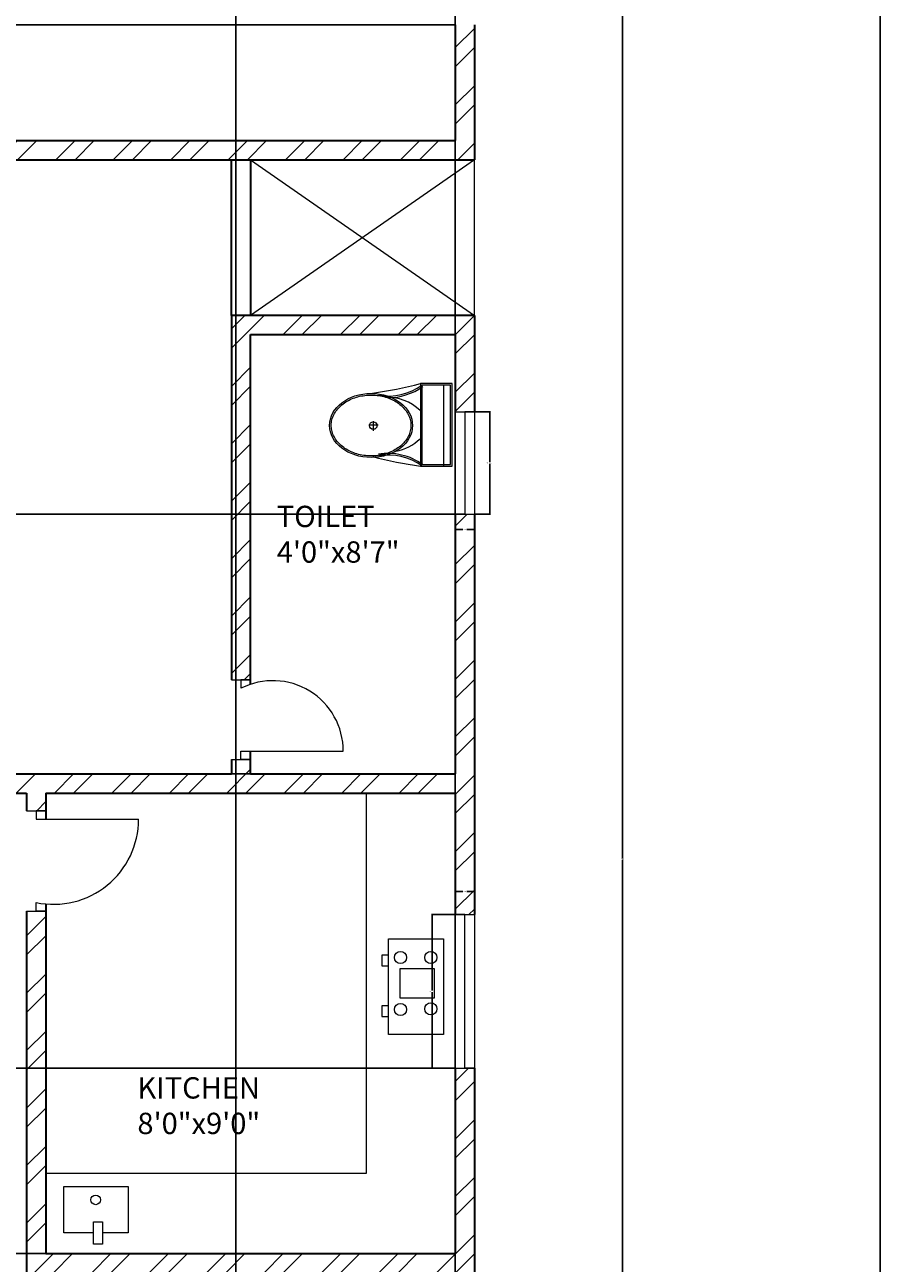
# Model space of a CAD drawing. Units: inches. Extents: x 1965 to 2673, y 1802 to 2669.
# Tile 15 of 16: x 2473 to 2673, y 2154 to 2444. Entities that reach past the tile are written whole.
import ezdxf

# ---------------------------------------------------------------- set-up
doc = ezdxf.new("R2010")
doc.units = ezdxf.units.IN
for name, color, linetype, lineweight in [('A-ANNO-DIMS', 2, 'Continuous', 18), ('A-ANNO-TTLB', 7, 'Continuous', 25), ('A-AREA-IDEN', 7, 'Continuous', 18), ('A-DOOR', 11, 'Continuous', 18), ('A-EQPM', 8, 'Continuous', 18), ('A-FLOR-CASE', 8, 'Continuous', 18), ('A-FLOR-FIXT', 9, 'Continuous', 18), ('A-FLOR-OPEN', 8, 'Continuous', 13), ('A-GLAZ', 181, 'Continuous', 18), ('A-WALL', 7, 'Continuous', 35), ('A-WALL-PATT', 252, 'Continuous', 13)]:
    doc.layers.add(name, color=color, linetype=linetype, lineweight=lineweight)
doc.styles.get("Standard").update_dxf_attribs({"font": 'arial.ttf'})
doc.dimstyles.get("Standard").update_dxf_attribs({"dimtxt": 0.18, "dimasz": 0.18, "dimexe": 0.18, "dimexo": 0.0625, "dimgap": 0.09, "dimtad": 0, "dimtih": 1, "dimtoh": 1, "dimdec": 4, "dimzin": 0, "dimdsep": 46, "dimtxsty": 'Standard', "dimcen": 0.09, "dimadec": 0, "dimazin": 0, "dimtfac": 1, "dimtdec": 4, "dimtofl": 0, "dimtmove": 0, "dimatfit": 3, "dimfxl": 1, "dimtolj": 1, "dimtzin": 0, "dimarcsym": 0})

# ---------------------------------------------------------------- blocks, each defined once
blk = doc.blocks.new('A$C31115884')
for p, q in [((283.1, 497.7), (223.4, 497.7)), ((257.5, 466.4), (257.5, 523.2)), ((0, 200), (0, 0)), ((520, 200), (0, 200)), ((10, 190), (10, 10)), ((510, 190), (10, 190)), ((510, 10), (510, 190)), ((520, 0), (520, 200)), ((510, 54.5), (0, 54.5)), ((10, 10), (510, 10)), ((0, 0), (520, 0))]:
    blk.add_line(p, q)
blk.add_circle((255.6, 496.4), 23.6)
for centre, radius, start, end in [((2777.7, -204.6), 2807, 165.4549, 171.71327), ((3237, 905), 2807, 188.28673, 194.5451), ((-294.5, 403.3), 364.7, 324.20913, 9.34987), ((-294.5, 403.3), 374.7, 324.20913, 9.34987), ((139.5, 406.2), 293.5, 315.84364, 2.65635), ((805.8, 403.3), 374.7, 179.20365, 215.79087), ((805.8, 403.3), 364.7, 170.65013, 215.79087), ((383.6, 406.2), 293.5, 190.27735, 224.15636)]:
    blk.add_arc(centre, radius, start, end)
blk.add_ellipse((256.2, 509.9), major_axis=(0, -260.7), ratio=0.772727)
blk.add_open_spline([(256.2, 259.2), (263.1, 259.2), (270, 259.7), (287.8, 262.3), (298.7, 265.1), (319.9, 273.1), (330.2, 278.4), (350.1, 291.1), (359.7, 298.7), (377.7, 315.9), (386.2, 325.5), (401.7, 346.6), (408.8, 358.1), (421.3, 382.5), (426.8, 395.5), (435.9, 422.4), (439.5, 436.4), (444.8, 465.1), (446.5, 479.7), (447.9, 509.2), (447.6, 524), (445, 553.3), (442.7, 567.8), (436.3, 596), (432.1, 609.7), (421.9, 636), (416, 648.6), (402.5, 672.1), (395, 683), (378.6, 703), (369.8, 712.1), (351.1, 728), (341.3, 734.8), (320.9, 746.2), (310.4, 750.7), (288.9, 757.3), (278, 759.4), (256, 761), (245, 760.6), (223.1, 757.2), (212.3, 754.3), (191.1, 746.1), (180.8, 740.7), (160.9, 727.8), (151.4, 720.1), (133.5, 702.7), (125.1, 693), (109.6, 671.7), (102.6, 660.2), (90.2, 635.7), (84.9, 622.7), (76, 595.6), (72.4, 581.6), (67.2, 552.9), (65.6, 538.2), (64.4, 508.8), (64.8, 494), (67.5, 464.7), (69.9, 450.2), (76.6, 422), (80.8, 408.3), (91.1, 382.2), (97.2, 369.7), (110.8, 346.3), (118.4, 335.4), (134.8, 315.6), (143.7, 306.7), (162.4, 290.9), (172.3, 284.2), (192.8, 273), (203.3, 268.6), (224.8, 262.2), (235.8, 260.2), (249.9, 259.3), (253, 259.2), (256.2, 259.2)], degree=3, knots=[0, 0, 0, 0, 0.110105, 0.110105, 0.285049, 0.285049, 0.459994, 0.459994, 0.634938, 0.634938, 0.809882, 0.809882, 0.984827, 0.984827, 1.159771, 1.159771, 1.334715, 1.334715, 1.50966, 1.50966, 1.684604, 1.684604, 1.859549, 1.859549, 2.034493, 2.034493, 2.209437, 2.209437, 2.384382, 2.384382, 2.559326, 2.559326, 2.73427, 2.73427, 2.909215, 2.909215, 3.084159, 3.084159, 3.259103, 3.259103, 3.434048, 3.434048, 3.608992, 3.608992, 3.783936, 3.783936, 3.958881, 3.958881, 4.133825, 4.133825, 4.30877, 4.30877, 4.483714, 4.483714, 4.658658, 4.658658, 4.833603, 4.833603, 5.008547, 5.008547, 5.183491, 5.183491, 5.358436, 5.358436, 5.53338, 5.53338, 5.708324, 5.708324, 5.883269, 5.883269, 6.058213, 6.058213, 6.233158, 6.233158, 6.283185, 6.283185, 6.283185, 6.283185])
blk = doc.blocks.new('WIN-24IN')
for p, q in [((0, 24), (4.5, 24)), ((0, 24), (0, 0)), ((4.5, 24), (2.25, 24)), ((2.25, 24), (2.25, 0)), ((4.5, 24), (4.5, 0)), ((2.25, 0), (0, 0)), ((0, 0), (4.5, 0))]:
    blk.add_line(p, q)
blk = doc.blocks.new('WIN-36IN')
for p, q in [((2.25, 36.01), (0, 36.01)), ((0, 36.01), (4.5, 36.01)), ((0, 36.01), (0, 0.01)), ((2.25, 0.01), (2.25, 36.01)), ((4.5, 36.01), (4.5, 0.01)), ((0, 0.01), (4.5, 0.01)), ((4.5, 0.01), (2.25, 0.01))]:
    blk.add_line(p, q)
blk = doc.blocks.new('SHAFT-OPENING')
for p, q in [((0, 36.5), (0, 0)), ((52.5, 0), (0, 36.5)), ((0, 0), (52.5, 36.5))]:
    blk.add_line(p, q)
blk = doc.blocks.new('*D11')
at = {"layer": 'A-ANNO-DIMS', "color": 0, "lineweight": -2, "transparency": 16777216}
for p, q in [((2578.16, 2353.47), (2581.87, 2353.47)), ((2581.69, 2353.29), (2581.69, 2341.65)), ((2581.69, 2329.65), (2581.69, 2341.29)), ((2578.16, 2329.47), (2581.87, 2329.47))]:
    blk.add_line(p, q, dxfattribs=at)
at = {"layer": 'A-ANNO-DIMS', "color": 0, "transparency": 16777216}
for points in [[(2581.66, 2353.29), (2581.72, 2353.29), (2581.69, 2353.47)], [(2581.66, 2329.65), (2581.72, 2329.65), (2581.69, 2329.47)]]:
    blk.add_solid(points, dxfattribs=at)
at = {"layer": 'Defpoints', "color": 0, "transparency": 16777216}
for p in [(2578.09, 2353.47), (2581.69, 2353.47), (2578.09, 2329.47)]:
    blk.add_point(p, dxfattribs=at)
at = {"layer": 'A-ANNO-DIMS', "color": 0, "transparency": 16777216, "insert": (2581.69, 2341.47), "char_height": 0.18, "attachment_point": 5}
blk.add_mtext('\\A1;WIN. 24 TYP.', dxfattribs=at)
blk = doc.blocks.new('*D12')
at = {"layer": 'A-ANNO-DIMS', "color": 0, "lineweight": -2, "transparency": 16777216}
for p, q in [((2573.59, 2329.4), (2573.59, 2325.69)), ((2578.09, 2329.4), (2578.09, 2325.69)), ((2573.77, 2325.87), (2575.38, 2325.87)), ((2577.91, 2325.87), (2576.3, 2325.87))]:
    blk.add_line(p, q, dxfattribs=at)
at = {"layer": 'A-ANNO-DIMS', "color": 0, "transparency": 16777216}
for points in [[(2573.77, 2325.9), (2573.77, 2325.84), (2573.59, 2325.87)], [(2577.91, 2325.9), (2577.91, 2325.84), (2578.09, 2325.87)]]:
    blk.add_solid(points, dxfattribs=at)
at = {"layer": 'Defpoints', "color": 0, "transparency": 16777216}
for p in [(2573.59, 2329.47), (2578.09, 2329.47), (2578.09, 2325.87)]:
    blk.add_point(p, dxfattribs=at)
at = {"layer": 'A-ANNO-DIMS', "color": 0, "transparency": 16777216, "insert": (2575.84, 2325.87), "char_height": 0.18, "attachment_point": 5}
blk.add_mtext('\\A1;5 TYP.', dxfattribs=at)
blk = doc.blocks.new('*D13')
at = {"layer": 'A-ANNO-DIMS', "color": 0, "lineweight": -2, "transparency": 16777216}
for p, q in [((2573.53, 2235.58), (2568.01, 2235.58)), ((2568.19, 2235.4), (2568.19, 2217.76)), ((2568.19, 2199.76), (2568.19, 2217.39)), ((2573.53, 2199.58), (2568.01, 2199.58))]:
    blk.add_line(p, q, dxfattribs=at)
at = {"layer": 'A-ANNO-DIMS', "color": 0, "transparency": 16777216}
for points in [[(2568.16, 2235.4), (2568.22, 2235.4), (2568.19, 2235.58)], [(2568.16, 2199.76), (2568.22, 2199.76), (2568.19, 2199.58)]]:
    blk.add_solid(points, dxfattribs=at)
at = {"layer": 'Defpoints', "color": 0, "transparency": 16777216}
for p in [(2568.19, 2235.58), (2573.59, 2235.58), (2573.59, 2199.58)]:
    blk.add_point(p, dxfattribs=at)
at = {"layer": 'A-ANNO-DIMS', "color": 0, "transparency": 16777216, "insert": (2568.19, 2217.58), "char_height": 0.18, "attachment_point": 5}
blk.add_mtext('\\A1;WIN. 36 TYP.', dxfattribs=at)
blk = doc.blocks.new('*D14')
at = {"layer": 'A-ANNO-DIMS', "color": 0, "lineweight": -2, "transparency": 16777216}
for p, q in [((2573.59, 2235.64), (2573.59, 2241.16)), ((2573.77, 2240.98), (2575.38, 2240.98)), ((2577.91, 2240.98), (2576.3, 2240.98)), ((2578.09, 2235.64), (2578.09, 2241.16))]:
    blk.add_line(p, q, dxfattribs=at)
at = {"layer": 'A-ANNO-DIMS', "color": 0, "transparency": 16777216}
for points in [[(2573.77, 2241.01), (2573.77, 2240.95), (2573.59, 2240.98)], [(2577.91, 2241.01), (2577.91, 2240.95), (2578.09, 2240.98)]]:
    blk.add_solid(points, dxfattribs=at)
at = {"layer": 'Defpoints', "color": 0, "transparency": 16777216}
for p in [(2578.09, 2240.98), (2573.59, 2235.58), (2578.09, 2235.58)]:
    blk.add_point(p, dxfattribs=at)
at = {"layer": 'A-ANNO-DIMS', "color": 0, "transparency": 16777216, "insert": (2575.84, 2240.98), "char_height": 0.18, "attachment_point": 5}
blk.add_mtext('\\A1;5 TYP.', dxfattribs=at)
blk = doc.blocks.new('*D26')
at = {"layer": 'A-ANNO-DIMS', "color": 0, "lineweight": -2, "transparency": 16777216}
for p, q in [((2578.16, 2565.59), (2613, 2565.59)), ((2612.82, 2565.41), (2612.82, 2248.77)), ((2612.82, 1931.77), (2612.82, 2248.41)), ((2578.16, 1931.59), (2613, 1931.59))]:
    blk.add_line(p, q, dxfattribs=at)
at = {"layer": 'A-ANNO-DIMS', "color": 0, "transparency": 16777216}
for points in [[(2612.79, 2565.41), (2612.85, 2565.41), (2612.82, 2565.59)], [(2612.79, 1931.77), (2612.85, 1931.77), (2612.82, 1931.59)]]:
    blk.add_solid(points, dxfattribs=at)
at = {"layer": 'Defpoints', "color": 0, "transparency": 16777216}
for p in [(2578.09, 2565.59), (2612.82, 2565.59), (2578.09, 1931.59)]:
    blk.add_point(p, dxfattribs=at)
at = {"layer": 'A-ANNO-DIMS', "color": 0, "transparency": 16777216, "insert": (2612.82, 2248.59), "char_height": 0.18, "attachment_point": 5}
blk.add_mtext('\\A1;634', dxfattribs=at)
blk = doc.blocks.new('*D44')
at = {"layer": 'A-ANNO-DIMS', "color": 0, "lineweight": -2, "transparency": 16777216}
for p, q in [((2522.13, 1936.15), (2522.13, 2600.5)), ((2522.31, 2600.32), (2547.47, 2600.32)), ((2573.41, 2600.32), (2548.26, 2600.32)), ((2573.59, 1936.15), (2573.59, 2600.5))]:
    blk.add_line(p, q, dxfattribs=at)
at = {"layer": 'A-ANNO-DIMS', "color": 0, "transparency": 16777216}
for points in [[(2522.31, 2600.35), (2522.31, 2600.29), (2522.13, 2600.32)], [(2573.41, 2600.35), (2573.41, 2600.29), (2573.59, 2600.32)]]:
    blk.add_solid(points, dxfattribs=at)
at = {"layer": 'Defpoints', "color": 0, "transparency": 16777216}
for p in [(2573.59, 2600.32), (2522.13, 1936.09), (2573.59, 1936.09)]:
    blk.add_point(p, dxfattribs=at)
at = {"layer": 'A-ANNO-DIMS', "color": 0, "transparency": 16777216, "insert": (2547.86, 2600.32), "char_height": 0.18, "attachment_point": 5}
blk.add_mtext('\\A1;51.46', dxfattribs=at)
blk = doc.blocks.new('*D47')
at = {"layer": 'A-ANNO-DIMS', "color": 0, "lineweight": -2, "transparency": 16777216}
for p, q in [((2573.53, 2199.58), (2012.19, 2199.58)), ((2012.37, 2199.4), (2012.37, 2178.02)), ((2012.37, 2156.27), (2012.37, 2177.65)), ((2573.53, 2156.09), (2012.19, 2156.09))]:
    blk.add_line(p, q, dxfattribs=at)
at = {"layer": 'A-ANNO-DIMS', "color": 0, "transparency": 16777216}
for points in [[(2012.34, 2199.4), (2012.4, 2199.4), (2012.37, 2199.58)], [(2012.34, 2156.27), (2012.4, 2156.27), (2012.37, 2156.09)]]:
    blk.add_solid(points, dxfattribs=at)
at = {"layer": 'Defpoints', "color": 0, "transparency": 16777216}
for p in [(2012.37, 2199.58), (2573.59, 2199.58), (2573.59, 2156.09)]:
    blk.add_point(p, dxfattribs=at)
at = {"layer": 'A-ANNO-DIMS', "color": 0, "transparency": 16777216, "insert": (2012.37, 2177.83), "char_height": 0.18, "attachment_point": 5}
blk.add_mtext('\\A1;43.48', dxfattribs=at)
blk = doc.blocks.new('*D48')
at = {"layer": 'A-ANNO-DIMS', "color": 0, "lineweight": -2, "transparency": 16777216}
for p, q in [((2573.53, 2329.47), (2012.19, 2329.47)), ((2012.37, 2329.29), (2012.37, 2299.21)), ((2012.37, 2268.77), (2012.37, 2298.85)), ((2573.53, 2268.59), (2012.19, 2268.59))]:
    blk.add_line(p, q, dxfattribs=at)
at = {"layer": 'A-ANNO-DIMS', "color": 0, "transparency": 16777216}
for points in [[(2012.34, 2329.29), (2012.4, 2329.29), (2012.37, 2329.47)], [(2012.34, 2268.77), (2012.4, 2268.77), (2012.37, 2268.59)]]:
    blk.add_solid(points, dxfattribs=at)
at = {"layer": 'Defpoints', "color": 0, "transparency": 16777216}
for p in [(2012.37, 2329.47), (2573.59, 2329.47), (2573.59, 2268.59)]:
    blk.add_point(p, dxfattribs=at)
at = {"layer": 'A-ANNO-DIMS', "color": 0, "transparency": 16777216, "insert": (2012.37, 2299.03), "char_height": 0.18, "attachment_point": 5}
blk.add_mtext('\\A1;60.87', dxfattribs=at)
blk = doc.blocks.new('*D49')
at = {"layer": 'A-ANNO-DIMS', "color": 0, "lineweight": -2, "transparency": 16777216}
for p, q in [((2573.53, 2444.23), (2012.19, 2444.23)), ((2012.37, 2444.05), (2012.37, 2430.84)), ((2012.37, 2417.27), (2012.37, 2430.48)), ((2573.53, 2417.09), (2012.19, 2417.09))]:
    blk.add_line(p, q, dxfattribs=at)
at = {"layer": 'A-ANNO-DIMS', "color": 0, "transparency": 16777216}
for points in [[(2012.34, 2444.05), (2012.4, 2444.05), (2012.37, 2444.23)], [(2012.34, 2417.27), (2012.4, 2417.27), (2012.37, 2417.09)]]:
    blk.add_solid(points, dxfattribs=at)
at = {"layer": 'Defpoints', "color": 0, "transparency": 16777216}
for p in [(2012.37, 2444.23), (2573.59, 2444.23), (2573.59, 2417.09)]:
    blk.add_point(p, dxfattribs=at)
at = {"layer": 'A-ANNO-DIMS', "color": 0, "transparency": 16777216, "insert": (2012.37, 2430.66), "char_height": 0.18, "attachment_point": 5}
blk.add_mtext('\\A1;27.137', dxfattribs=at)

msp = doc.modelspace()

# ---------------------------------------------------------------- hatches: boundary and pattern name
at = {"layer": 'A-WALL-PATT'}
h = msp.add_hatch(dxfattribs=at)
h.set_pattern_fill('ANSI32', color=256)
h.paths.add_polyline_path([(2051.5927, 2561.0914), (2076.7559, 2561.0914), (2076.7559, 2563.3414), (2076.7559, 2565.5914), (2047.0927, 2565.5914), (2047.0927, 2518.3824), (2051.5927, 2518.3824)])
h.paths.add_polyline_path([(2051.5927, 2458.3824), (2049.3427, 2458.3824), (2047.0927, 2458.3824), (2047.0927, 2412.5914), (2248.0927, 2412.5914), (2248.0927, 2268.5914), (2252.5927, 2268.5914), (2252.5927, 2412.5914), (2252.5927, 2421.0404), (2250.3427, 2421.0404), (2248.0927, 2421.0404), (2248.0927, 2417.0914), (2051.5927, 2417.0914)])
h.paths.add_polyline_path([(2211.4933, 2268.5914), (2104.0927, 2268.5914), (2104.0927, 2272.4654), (2101.8427, 2272.4654), (2099.5927, 2272.4654), (2099.5927, 2268.5914), (2051.5927, 2268.5914), (2051.5927, 2264.0914), (2147.5927, 2264.0914), (2147.5927, 2259.8893), (2152.0927, 2259.8893), (2152.0927, 2264.0914), (2211.4933, 2264.0914), (2211.4933, 2266.3414)])
h.paths.add_polyline_path([(2104.0927, 2376.0914), (2099.5927, 2376.0914), (2047.0927, 2376.0914), (2047.0927, 2333.0682), (2051.5927, 2333.0682), (2051.5927, 2371.5914), (2099.5927, 2371.5914), (2099.5927, 2293.6123), (2104.0927, 2293.6123)], flags=17)
h.paths.add_polyline_path([(2051.5927, 2309.0682), (2047.0927, 2309.0682), (2047.0927, 2233.5821), (2051.5927, 2233.5821)])
h.paths.add_polyline_path([(2104.0927, 2412.5914), (2099.5927, 2412.5914), (2099.5927, 2376.0914), (2104.0927, 2376.0914)], flags=17)
h.paths.add_polyline_path([(2290.1254, 2268.5914), (2242.4924, 2268.5914), (2242.4924, 2264.0914), (2290.1254, 2264.0914), (2290.1254, 2266.3414)])
h.paths.add_polyline_path([(2284.653, 2264.0914), (2280.153, 2264.0914), (2280.153, 2161.6826), (2284.653, 2161.6826)])
h.paths.add_polyline_path([(2578.0927, 2329.4656), (2573.5927, 2329.4656), (2573.5927, 2268.5914), (2525.5927, 2268.5914), (2525.5927, 2271.9222), (2523.3427, 2271.9222), (2521.0927, 2271.9222), (2521.0927, 2268.5914), (2324.2835, 2268.5914), (2324.2835, 2264.0914), (2329.0927, 2264.0914), (2329.0927, 2259.4977), (2333.5927, 2259.4977), (2333.5927, 2264.0914), (2473.0927, 2264.0914), (2473.0927, 2259.9371), (2477.5927, 2259.9371), (2477.5927, 2264.0914), (2573.5927, 2264.0914), (2573.5927, 2235.5751), (2578.0927, 2235.5751)])
h.paths.add_polyline_path([(2377.0927, 2412.5914), (2578.0927, 2412.5914), (2578.0927, 2444.2286), (2575.8427, 2444.2286), (2573.5927, 2444.2286), (2573.5927, 2417.0914), (2429.5927, 2417.0914), (2377.0927, 2417.0914), (2377.0927, 2421.7443), (2372.5927, 2421.7443), (2372.5927, 2268.5914), (2377.0927, 2268.5914)])
h.paths.add_polyline_path([(2525.5927, 2371.5914), (2573.5927, 2371.5914), (2573.5927, 2353.4656), (2578.0927, 2353.4656), (2578.0927, 2376.0914), (2525.5927, 2376.0914), (2521.0927, 2376.0914), (2521.0927, 2290.6472), (2525.5927, 2290.6472)], flags=17)
h.paths.add_polyline_path([(2477.5927, 2236.4106), (2475.3427, 2236.4106), (2473.0927, 2236.4106), (2473.0927, 2084.5914), (2465.3309, 2084.5914), (2465.3309, 2080.0914), (2481.6764, 2080.0914), (2481.6764, 2082.3414), (2481.6764, 2084.5914), (2477.5927, 2084.5914), (2477.5927, 2151.5914), (2573.5927, 2151.5914), (2573.5927, 2130.2907), (2578.0927, 2130.2907), (2578.0927, 2199.5751), (2575.8427, 2199.5751), (2573.5927, 2199.5751), (2573.5927, 2156.0914), (2477.5927, 2156.0914)])
h.paths.add_polyline_path([(2573.5927, 2084.5914), (2505.5513, 2084.5914), (2505.5513, 2080.0914), (2573.5927, 2080.0914)], flags=17)
h.paths.add_polyline_path([(2578.0927, 2106.2907), (2575.8427, 2106.2907), (2573.5927, 2106.2907), (2573.5927, 2050.8986), (2578.0927, 2050.8986)])
h.paths.add_polyline_path([(2578.0927, 1990.8986), (2575.8427, 1990.8986), (2573.5927, 1990.8986), (2573.5927, 1936.0914), (2522.132, 1936.0914), (2522.132, 1931.5914), (2578.0927, 1931.5914)])
h.paths.add_polyline_path([(2462.132, 1936.0914), (2429.5927, 1936.0914), (2429.5927, 2080.0914), (2432.623, 2080.0914), (2432.623, 2082.3414), (2432.623, 2084.5914), (2429.5927, 2084.5914), (2429.5927, 2120.5914), (2333.5927, 2120.5914), (2333.5927, 2229.3125), (2331.3427, 2229.3125), (2329.0927, 2229.3125), (2329.0927, 2116.0914), (2425.0927, 2116.0914), (2425.0927, 1936.0914), (2346.4058, 1936.0914), (2346.4058, 1931.5914), (2462.132, 1931.5914), (2462.132, 1933.8414)])
h.paths.add_polyline_path([(2211.767, 1933.8414), (2211.767, 1936.0914), (2200.0927, 1936.0914), (2200.0927, 2080.0914), (2200.0927, 2116.0914), (2284.653, 2116.0914), (2284.653, 2130.591), (2282.403, 2130.591), (2280.153, 2130.591), (2280.153, 2120.5914), (2200.0927, 2120.5914), (2195.5927, 2120.5914), (2195.5927, 2080.0914), (2195.5927, 1936.0914), (2139.0533, 1936.0914), (2139.0533, 1931.5914), (2211.767, 1931.5914)])
h.paths.add_polyline_path([(2282.2502, 1933.8414), (2282.2502, 1936.0914), (2259.767, 1936.0914), (2259.767, 1931.5914), (2282.2502, 1931.5914)], flags=17)
h.paths.add_polyline_path([(2051.5927, 1987.096), (2049.3427, 1987.096), (2047.0927, 1987.096), (2047.0927, 1931.5914), (2079.0533, 1931.5914), (2079.0533, 1933.8414), (2079.0533, 1936.0914), (2051.5927, 1936.0914)])
h.paths.add_polyline_path([(2051.5927, 2197.5821), (2049.3427, 2197.5821), (2047.0927, 2197.5821), (2047.0927, 2141.952), (2051.5927, 2141.952), (2051.5927, 2151.5914), (2147.5927, 2151.5914), (2147.5927, 2084.5914), (2144.3652, 2084.5914), (2144.3652, 2080.0914), (2155.9662, 2080.0914), (2155.9662, 2082.3414), (2155.9662, 2084.5914), (2152.0927, 2084.5914), (2152.0927, 2239.4921), (2149.8427, 2239.4921), (2147.5927, 2239.4921), (2147.5927, 2156.0914), (2051.5927, 2156.0914)])
h.paths.add_polyline_path([(2051.5927, 2080.0914), (2123.8575, 2080.0914), (2123.8575, 2082.3414), (2123.8575, 2084.5914), (2051.5927, 2084.5914), (2051.5927, 2117.952), (2047.0927, 2117.952), (2047.0927, 2047.096), (2051.5927, 2047.096)])
h = msp.add_hatch(dxfattribs=at)
h.set_pattern_fill('ANSI32', color=256)
h.paths.add_polyline_path([(2210.2316, 2563.3414), (2210.2316, 2565.5914), (2136.7559, 2565.5914), (2136.7559, 2561.0914), (2195.5927, 2561.0914), (2195.5927, 2485.8604), (2200.0927, 2485.8604), (2200.0927, 2561.0914), (2210.2316, 2561.0914)])
h.paths.add_polyline_path([(2285.9734, 2565.5914), (2234.2316, 2565.5914), (2234.2316, 2561.0914), (2248.0927, 2561.0914), (2248.0927, 2462.0914), (2200.0927, 2462.0914), (2200.0927, 2465.2357), (2197.8427, 2465.2357), (2195.5927, 2465.2357), (2195.5927, 2457.5914), (2248.0927, 2457.5914), (2248.0927, 2452.628), (2252.5927, 2452.628), (2252.5927, 2457.5914), (2257.5156, 2457.5914), (2257.5156, 2459.8414), (2257.5156, 2462.0914), (2252.5927, 2462.0914), (2252.5927, 2561.0914), (2285.9734, 2561.0914)])
h.paths.add_polyline_path([(2213.1374, 1872.8885), (2461.061, 1872.8885), (2461.061, 1909.9813), (2213.1374, 1909.9813)], flags=9)
h.paths.add_polyline_path([(2328.4056, 1942.3944), (2340.6089, 1942.3944), (2340.6089, 1952.6979), (2328.4056, 1952.6979)], flags=9)
h.paths.add_polyline_path([(2353.5759, 2030.9808), (2376.6455, 2030.9808), (2376.6455, 2041.2844), (2353.5759, 2041.2844)], flags=9)
h.paths.add_polyline_path([(2289.989, 2074.1041), (2326.916, 2074.1041), (2326.916, 2092.7615), (2289.989, 2092.7615)], flags=9)
h.paths.add_polyline_path([(2497.9, 2052.8638), (2548.3741, 2052.8638), (2548.3741, 2071.5212), (2497.9, 2071.5212)], flags=9)
h.paths.add_polyline_path([(2486.59, 2116.4883), (2515.7475, 2116.4883), (2515.7475, 2135.1456), (2486.59, 2135.1456)], flags=9)
h.paths.add_polyline_path([(2497.3007, 2181.2877), (2530.459, 2181.2877), (2530.459, 2199.945), (2497.3007, 2199.945)], flags=9)
h.paths.add_polyline_path([(2288.237, 2190.3228), (2324.1238, 2190.3228), (2324.1238, 2208.9802), (2288.237, 2208.9802)], flags=9)
h.paths.add_polyline_path([(2350.806, 2127.8307), (2387.733, 2127.8307), (2387.733, 2146.488), (2350.806, 2146.488)], flags=9)
h.paths.add_polyline_path([(2530.3237, 2315.2679), (2559.5563, 2315.2679), (2559.5563, 2333.9252), (2530.3237, 2333.9252)], flags=9)
h.paths.add_polyline_path([(2418.419, 2383.4707), (2468.2894, 2383.4707), (2468.2894, 2402.1281), (2418.419, 2402.1281)], flags=9)
h.paths.add_polyline_path([(2327.4503, 2399.0281), (2364.3773, 2399.0281), (2364.3773, 2417.6854), (2327.4503, 2417.6854)], flags=9)
h.paths.add_polyline_path([(2147.9722, 2271.4601), (2197.8426, 2271.4601), (2197.8426, 2290.1174), (2147.9722, 2290.1174)], flags=9)
h.paths.add_polyline_path([(2474.3875, 2421.594), (2524.8616, 2421.594), (2524.8616, 2440.2514), (2474.3875, 2440.2514)], flags=9)
h.paths.add_polyline_path([(2063.9863, 2052.9059), (2114.4604, 2052.9059), (2114.4604, 2071.5632), (2063.9863, 2071.5632)], flags=9)
h.paths.add_polyline_path([(2200.3335, 2133.7067), (2237.2605, 2133.7067), (2237.2605, 2152.364), (2200.3335, 2152.364)], flags=9)
h.paths.add_polyline_path([(2080.5973, 2184.636), (2113.8681, 2184.636), (2113.8681, 2203.2933), (2080.5973, 2203.2933)], flags=9)
h.paths.add_polyline_path([(2102.4918, 2116.4497), (2131.6494, 2116.4497), (2131.6494, 2135.107), (2102.4918, 2135.107)], flags=9)
h.paths.add_polyline_path([(2056.2753, 2308.5576), (2085.5079, 2308.5576), (2085.5079, 2327.2149), (2056.2753, 2327.2149)], flags=9)
h.paths.add_polyline_path([(2385.619, 2500.9729), (2414.8516, 2500.9729), (2414.8516, 2519.6303), (2385.619, 2519.6303)], flags=9)
h.paths.add_polyline_path([(2286.6643, 2508.6826), (2320.0715, 2508.6826), (2320.0715, 2527.34), (2286.6643, 2527.34)], flags=9)
h.paths.add_polyline_path([(2206.5604, 2500.7243), (2235.793, 2500.7243), (2235.793, 2519.3817), (2206.5604, 2519.3817)], flags=25)
h.paths.add_polyline_path([(2062.6644, 2424.4027), (2112.5348, 2424.4027), (2112.5348, 2443.0601), (2062.6644, 2443.0601)], flags=9)
h = msp.add_hatch(dxfattribs=at)
h.set_pattern_fill('ANSI32', color=256)
h.paths.add_polyline_path([(2429.5927, 2468.6101), (2427.3427, 2468.6101), (2425.0927, 2468.6101), (2425.0927, 2462.0914), (2377.0927, 2462.0914), (2377.0927, 2561.0914), (2390.4173, 2561.0914), (2390.4173, 2565.5914), (2321.9734, 2565.5914), (2321.9734, 2561.0914), (2372.5927, 2561.0914), (2372.5927, 2462.0914), (2281.6605, 2462.0914), (2281.6605, 2457.5914), (2372.5927, 2457.5914), (2372.5927, 2451.3316), (2377.0927, 2451.3316), (2377.0927, 2457.5914), (2429.5927, 2457.5914)])
h.paths.add_polyline_path([(2480.8929, 2565.5914), (2414.4173, 2565.5914), (2414.4173, 2561.0914), (2425.0927, 2561.0914), (2425.0927, 2489.9153), (2429.5927, 2489.9153), (2429.5927, 2561.0914), (2480.8929, 2561.0914), (2480.8929, 2563.3414)])
h.paths.add_polyline_path([(2213.1374, 1872.8885), (2461.061, 1872.8885), (2461.061, 1909.9813), (2213.1374, 1909.9813)], flags=9)
h.paths.add_polyline_path([(2328.4056, 1942.3944), (2340.6089, 1942.3944), (2340.6089, 1952.6979), (2328.4056, 1952.6979)], flags=9)
h.paths.add_polyline_path([(2353.5759, 2030.9808), (2376.6455, 2030.9808), (2376.6455, 2041.2844), (2353.5759, 2041.2844)], flags=9)
h.paths.add_polyline_path([(2289.989, 2074.1041), (2326.916, 2074.1041), (2326.916, 2092.7615), (2289.989, 2092.7615)], flags=9)
h.paths.add_polyline_path([(2497.9, 2052.8638), (2548.3741, 2052.8638), (2548.3741, 2071.5212), (2497.9, 2071.5212)], flags=9)
h.paths.add_polyline_path([(2486.59, 2116.4883), (2515.7475, 2116.4883), (2515.7475, 2135.1456), (2486.59, 2135.1456)], flags=9)
h.paths.add_polyline_path([(2497.3007, 2181.2877), (2530.459, 2181.2877), (2530.459, 2199.945), (2497.3007, 2199.945)], flags=9)
h.paths.add_polyline_path([(2288.237, 2190.3228), (2324.1238, 2190.3228), (2324.1238, 2208.9802), (2288.237, 2208.9802)], flags=9)
h.paths.add_polyline_path([(2350.806, 2127.8307), (2387.733, 2127.8307), (2387.733, 2146.488), (2350.806, 2146.488)], flags=9)
h.paths.add_polyline_path([(2530.3237, 2315.2679), (2559.5563, 2315.2679), (2559.5563, 2333.9252), (2530.3237, 2333.9252)], flags=9)
h.paths.add_polyline_path([(2418.419, 2383.4707), (2468.2894, 2383.4707), (2468.2894, 2402.1281), (2418.419, 2402.1281)], flags=9)
h.paths.add_polyline_path([(2327.4503, 2399.0281), (2364.3773, 2399.0281), (2364.3773, 2417.6854), (2327.4503, 2417.6854)], flags=9)
h.paths.add_polyline_path([(2147.9722, 2271.4601), (2197.8426, 2271.4601), (2197.8426, 2290.1174), (2147.9722, 2290.1174)], flags=9)
h.paths.add_polyline_path([(2474.3875, 2421.594), (2524.8616, 2421.594), (2524.8616, 2440.2514), (2474.3875, 2440.2514)], flags=9)
h.paths.add_polyline_path([(2063.9863, 2052.9059), (2114.4604, 2052.9059), (2114.4604, 2071.5632), (2063.9863, 2071.5632)], flags=9)
h.paths.add_polyline_path([(2200.3335, 2133.7067), (2237.2605, 2133.7067), (2237.2605, 2152.364), (2200.3335, 2152.364)], flags=9)
h.paths.add_polyline_path([(2080.5973, 2184.636), (2113.8681, 2184.636), (2113.8681, 2203.2933), (2080.5973, 2203.2933)], flags=9)
h.paths.add_polyline_path([(2102.4918, 2116.4497), (2131.6494, 2116.4497), (2131.6494, 2135.107), (2102.4918, 2135.107)], flags=9)
h.paths.add_polyline_path([(2056.2753, 2308.5576), (2085.5079, 2308.5576), (2085.5079, 2327.2149), (2056.2753, 2327.2149)], flags=9)
h.paths.add_polyline_path([(2385.619, 2500.9729), (2414.8516, 2500.9729), (2414.8516, 2519.6303), (2385.619, 2519.6303)], flags=25)
h.paths.add_polyline_path([(2286.6643, 2508.6826), (2320.0715, 2508.6826), (2320.0715, 2527.34), (2286.6643, 2527.34)], flags=25)
h.paths.add_polyline_path([(2206.5604, 2500.7243), (2235.793, 2500.7243), (2235.793, 2519.3817), (2206.5604, 2519.3817)], flags=9)
h.paths.add_polyline_path([(2062.6644, 2424.4027), (2112.5348, 2424.4027), (2112.5348, 2443.0601), (2062.6644, 2443.0601)], flags=9)

# ---------------------------------------------------------------- linework, layer by layer
at = {"layer": 'A-ANNO-TTLB'}
msp.add_lwpolyline([(1964.5703, 2669.282), (2673.2605, 2669.282), (2673.2605, 1802.0221), (1964.5703, 1802.0221)], close=True, dxfattribs=at)
at = {"layer": 'A-DOOR'}
for p, q in [((2521.0927, 2290.6472), (2525.5927, 2290.6472)), ((2525.5927, 2290.6472), (2523.3427, 2290.6472)), ((2523.3427, 2290.6472), (2523.3427, 2288.6472)), ((2523.3427, 2271.9222), (2523.3427, 2273.9222)), ((2523.3427, 2273.9222), (2547.3427, 2273.9222)), ((2521.0927, 2271.9222), (2525.5927, 2271.9222)), ((2525.5927, 2271.9222), (2523.3427, 2271.9222)), ((2473.0927, 2259.9371), (2477.5927, 2259.9371)), ((2477.5927, 2259.9371), (2475.3427, 2259.9371)), ((2475.3427, 2259.9371), (2475.3427, 2257.9371)), ((2475.3427, 2257.9371), (2499.3427, 2257.9371)), ((2473.0927, 2236.4106), (2477.5927, 2236.4106)), ((2475.3427, 2236.4106), (2475.3427, 2238.4106)), ((2477.5927, 2236.4106), (2475.3427, 2236.4106))]:
    msp.add_line(p, q, dxfattribs=at)
for centre, radius, start, end in [((2530.8255, 2273.9222), 16.5172, 0, 116.938392), ((2479.3993, 2257.9371), 19.9434, 258.263942, 0)]:
    msp.add_arc(centre, radius, start, end, dxfattribs=at)
at = {"layer": 'A-EQPM'}
for points in [[(2557.9186, 2229.9357), (2570.867, 2229.9357), (2570.867, 2207.4472), (2557.9186, 2207.4472)], [(2557.9186, 2226.0982), (2556.4054, 2226.0982), (2556.4054, 2223.5662), (2557.9186, 2223.5662)], [(2560.7021, 2222.9423), (2568.6333, 2222.9423), (2568.6333, 2215.9974), (2560.7021, 2215.9974)], [(2557.9186, 2214.2166), (2556.4054, 2214.2166), (2556.4054, 2211.6846), (2557.9186, 2211.6846)]]:
    msp.add_lwpolyline(points, close=True, dxfattribs=at)
for centre in [(2560.7656, 2225.511), (2567.872, 2225.511), (2560.7656, 2213.3336), (2567.872, 2213.4922)]:
    msp.add_circle(centre, 1.4271, dxfattribs=at)
at = {"layer": 'A-FLOR-CASE'}
for p, q in [((2552.7969, 2174.9208), (2552.7969, 2264.0914)), ((2477.5927, 2174.9208), (2552.7969, 2174.9208))]:
    msp.add_line(p, q, dxfattribs=at)
at = {"layer": 'A-FLOR-FIXT'}
msp.add_lwpolyline([(2488.7485, 2160.9845), (2481.8241, 2160.9845), (2481.8241, 2171.8249), (2496.8949, 2171.8249), (2496.8949, 2160.9845), (2490.9053, 2160.9845)], dxfattribs=at)
msp.add_lwpolyline([(2488.7485, 2163.5292), (2490.9053, 2163.5292), (2490.9053, 2158.2837), (2488.7485, 2158.2837)], close=True, dxfattribs=at)
msp.add_circle((2489.2917, 2168.6981), 1.1357, dxfattribs=at)
at = {"layer": 'A-GLAZ'}
for p, q in [((2573.5927, 2353.4656), (2573.5927, 2353.4656)), ((2573.5927, 2353.4656), (2573.5927, 2353.4656)), ((2578.0927, 2353.4656), (2578.0927, 2353.4656))]:
    msp.add_line(p, q, dxfattribs=at)
at = {"layer": 'A-WALL'}
for p, q in [((2573.5927, 2444.2286), (2573.5927, 2417.0914)), ((2578.0927, 2444.2286), (2578.0927, 2412.5914)), ((2377.0927, 2417.0914), (2573.5927, 2417.0914)), ((2429.5927, 2417.0914), (2573.5927, 2417.0914)), ((2377.0927, 2412.5914), (2578.0927, 2412.5914)), ((2521.0927, 2376.0914), (2521.0927, 2412.5914)), ((2521.0927, 2412.5914), (2525.5927, 2412.5914)), ((2525.5927, 2412.5914), (2525.5927, 2376.0914)), ((2525.5927, 2376.0914), (2521.0927, 2376.0914)), ((2521.0927, 2376.0914), (2521.0927, 2290.6472)), ((2521.0927, 2376.0914), (2521.0927, 2376.0914)), ((2578.0927, 2376.0914), (2525.5927, 2376.0914)), ((2578.0927, 2376.0914), (2578.0927, 2353.4656)), ((2525.5927, 2371.5914), (2573.5927, 2371.5914)), ((2525.5927, 2289.5886), (2525.5927, 2371.5914)), ((2573.5927, 2371.5914), (2573.5927, 2353.4656)), ((2573.5927, 2329.4656), (2573.5927, 2268.5914)), ((2578.0927, 2329.4656), (2578.0927, 2235.5751)), ((2525.5927, 2268.5914), (2525.5927, 2273.9222)), ((2521.0927, 2271.9222), (2521.0927, 2268.5914)), ((2322.5984, 2268.5914), (2521.0927, 2268.5914)), ((2525.5927, 2268.5914), (2573.5927, 2268.5914)), ((2333.5927, 2264.0914), (2473.0927, 2264.0914)), ((2473.0927, 2264.0914), (2473.0927, 2259.9371)), ((2477.5927, 2264.0914), (2477.5927, 2257.9371)), ((2477.5927, 2264.0914), (2573.5927, 2264.0914)), ((2573.5927, 2264.0914), (2573.5927, 2235.5751)), ((2473.0927, 2236.4106), (2473.0927, 2084.5914)), ((2477.5927, 2238.0757), (2477.5927, 2156.0914)), ((2573.5927, 2199.5751), (2573.5927, 2156.0914)), ((2578.0927, 2199.5751), (2578.0927, 2130.2907)), ((2477.5927, 2156.0914), (2573.5927, 2156.0914))]:
    msp.add_line(p, q, dxfattribs=at)

# ---------------------------------------------------------------- block references
at = {"layer": 'A-FLOR-FIXT', "xscale": 0.0372717239612423, "yscale": 0.0372717239612423, "zscale": 0.0372717239612423, "rotation": 89.99999999999999}
msp.add_blockref('A$C31115884', (2572.8718, 2340.7279), dxfattribs=at)
at = {"layer": 'A-FLOR-OPEN', "rotation": 180}
msp.add_blockref('SHAFT-OPENING', (2578.0954, 2412.5927), dxfattribs=at)
at = {"layer": 'A-GLAZ'}
for name, p in [('WIN-24IN', (2573.59, 2329.47)), ('WIN-36IN', (2573.59, 2199.57))]:
    msp.add_blockref(name, p, dxfattribs=at)

# ---------------------------------------------------------------- texts
at = {"layer": 'A-AREA-IDEN', "char_height": 5, "attachment_point": 1}
for s, width, insert in [('TOILET\\P4\'0"x8\'7"', 256.959746, (2531.7374, 2331.4406)), ('KITCHEN\\P8\'0"x9\'0"', 191.106626, (2499.0623, 2197.457))]:
    msp.add_mtext_dynamic_manual_height_columns(s, width=width, gutter_width=12.5, heights=[0], dxfattribs=dict(at, insert=insert))

# ---------------------------------------------------------------- dimensions: what is measured, and where the dimension line sits
at = {"layer": 'A-ANNO-DIMS'}
dim = msp.add_linear_dim(base=(2573.5927, 2600.3164), p1=(2522.132, 1936.0914), p2=(2573.5927, 1936.0914), dimstyle='Standard', override={"dimdec": 2, "dimlfac": 1, "dimrnd": 0, "dimzin": 0, "dimdsep": 46, "dimlunit": 2}, dxfattribs=at)
dim.commit()
dim.dimension.update_dxf_attribs({"geometry": '*D44', "text_midpoint": (2547.8623, 2600.3164)})
for base, p1, p2, override, picture, middle in [((2612.8177, 2565.5914), (2578.0927, 1931.5914), (2578.0927, 2565.5914), {"dimdec": 0, "dimlfac": 1, "dimrnd": 0, "dimzin": 0, "dimdsep": 46, "dimlunit": 2}, '*D26', (2612.8177, 2248.5914)), ((2012.3677, 2444.2286), (2573.5927, 2417.0914), (2573.5927, 2444.2286), {"dimdec": 3, "dimlfac": 1, "dimrnd": 0, "dimzin": 0, "dimdsep": 46, "dimlunit": 2}, '*D49', (2012.3677, 2430.66)), ((2012.3677, 2329.4656), (2573.5927, 2268.5914), (2573.5927, 2329.4656), {"dimdec": 2, "dimlfac": 1, "dimrnd": 0, "dimzin": 0, "dimdsep": 46, "dimlunit": 2}, '*D48', (2012.3677, 2299.0285)), ((2012.3677, 2199.5751), (2573.5927, 2156.0914), (2573.5927, 2199.5751), {"dimdec": 2, "dimlfac": 1, "dimrnd": 0, "dimzin": 0, "dimdsep": 46, "dimlunit": 2}, '*D47', (2012.3677, 2177.8332))]:
    dim = msp.add_linear_dim(base=base, p1=p1, p2=p2, angle=90, dimstyle='Standard', override=override, dxfattribs=at)
    dim.commit()
    dim.dimension.update_dxf_attribs({"geometry": picture, "text_midpoint": middle})
for base, p1, p2, picture, middle in [((2581.6927, 2353.4656), (2578.0927, 2329.4656), (2578.0927, 2353.4656), '*D11', (2581.6927, 2341.4656)), ((2568.1927, 2235.5751), (2573.5927, 2199.5751), (2573.5927, 2235.5751), '*D13', (2568.1927, 2217.5751))]:
    dim = msp.add_linear_dim(base=base, p1=p1, p2=p2, angle=90, text='WIN. <> TYP.', dimstyle='Standard', override={"dimdec": 0, "dimlfac": 1, "dimrnd": 0, "dimzin": 0, "dimdsep": 46, "dimlunit": 2}, dxfattribs=at)
    dim.commit()
    dim.dimension.update_dxf_attribs({"geometry": picture, "text_midpoint": middle})
for base, p1, p2, picture, middle in [((2578.0927007574, 2325.8656489963), (2573.5927007574, 2329.4656489963), (2578.0927007574, 2329.4656489963), '*D12', (2575.8427007574, 2325.8656489963)), ((2578.0927007574, 2240.9750652316), (2573.5927007574, 2235.5750652316), (2578.0927007574, 2235.5750652316), '*D14', (2575.8427007574, 2240.9750652316))]:
    dim = msp.add_linear_dim(base=base, p1=p1, p2=p2, text='<> TYP.', dimstyle='Standard', override={"dimdec": 0, "dimlfac": 1, "dimrnd": 0, "dimzin": 0, "dimdsep": 46, "dimlunit": 2}, dxfattribs=at)
    dim.commit()
    dim.dimension.update_dxf_attribs({"geometry": picture, "text_midpoint": middle})

doc.saveas('drawing.dxf')
